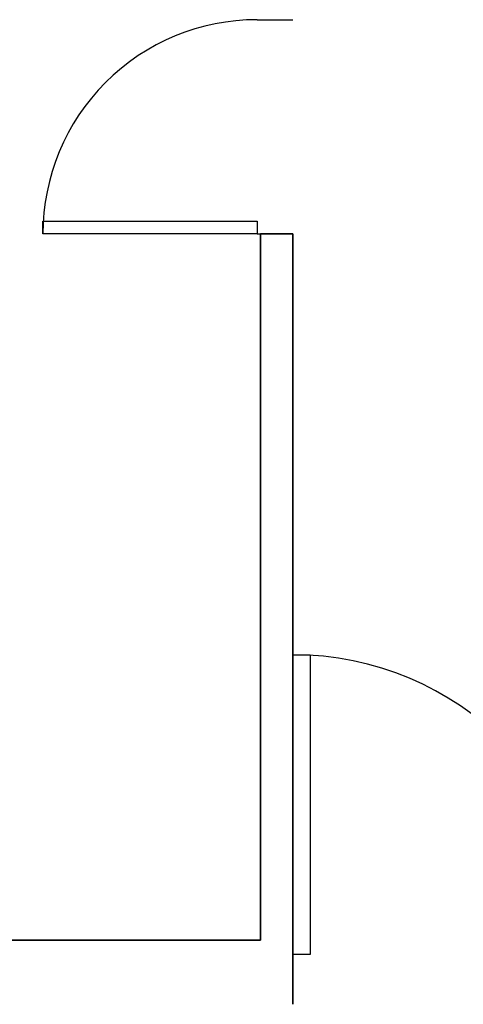
# Model space of a CAD drawing. Units: inches. Extents: x 108 to 613, y 1573 to 2319.
# Tile 3 of 11: x 261 to 323, y 1989 to 2127. Entities that reach past the tile are written whole.
import ezdxf

# ---------------------------------------------------------------- set-up
doc = ezdxf.new("R2010")
doc.units = ezdxf.units.IN
doc.layers.add('door', color=4, linetype='Continuous', lineweight=25)
doc.layers.add('wall', color=6, linetype='Continuous', lineweight=35)

# ---------------------------------------------------------------- blocks, each defined once
blk = doc.blocks.new('*U2')
for p, q in [((0, 0), (0, -5)), ((30, 0), (30, -5))]:
    blk.add_line(p, q)
blk.add_lwpolyline([(0, 0), (0, 30), (1.75, 30), (1.75, 0)], close=True)
blk.add_arc((0, 0), 30, 0, 90)

msp = doc.modelspace()

# ---------------------------------------------------------------- linework, layer by layer
at = {"layer": 'wall'}
for p, q in [((294.7753, 2096.6125), (299.2753, 2096.6125)), ((294.7753, 2096.6125), (294.7753, 1997.6125)), ((299.2753, 2096.6125), (299.2753, 1988.6125)), ((153.7753, 1997.6125), (294.7753, 1997.6125))]:
    msp.add_line(p, q, dxfattribs=at)

# ---------------------------------------------------------------- block references
at = {"layer": 'door', "rotation": 89.99999999999991}
msp.add_blockref('*U2', (294.2753, 2096.6125), dxfattribs=at)
at = {"layer": 'door', "xscale": 1.399999999999996, "yscale": 1.399999999999996, "zscale": 1.399999999999996}
msp.add_blockref('*U2', (299.2753, 1995.6125), dxfattribs=at)

doc.saveas('drawing.dxf')
